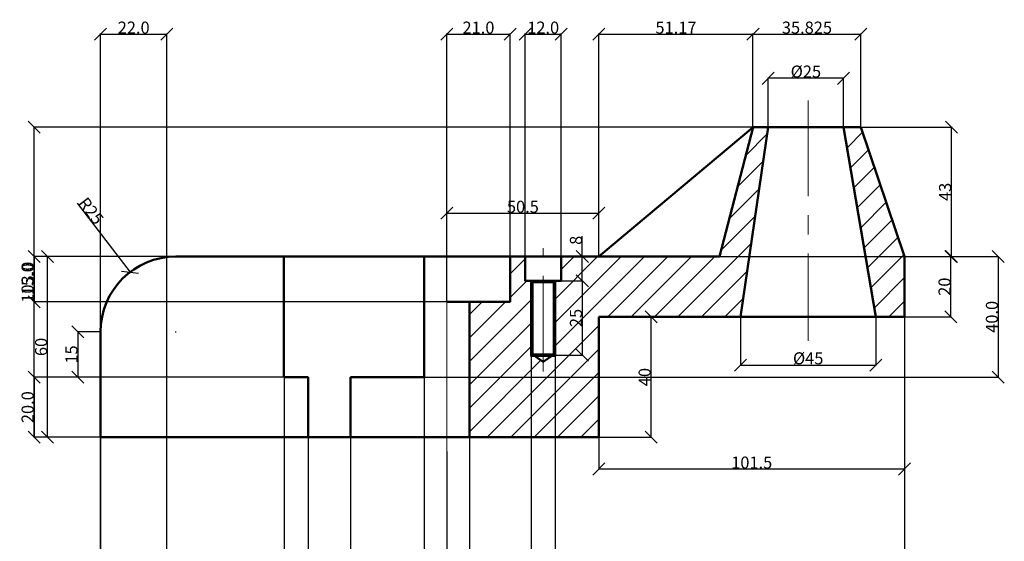
# Model space of a CAD drawing. Units: millimetres. Extents: x 263 to 611, y 50 to 522.
# Tile 5 of 5: x 284 to 611, y 349 to 522. Entities that reach past the tile are written whole.
import ezdxf

# ---------------------------------------------------------------- set-up
doc = ezdxf.new("R2010")
doc.units = ezdxf.units.MM
doc.header["$MEASUREMENT"] = 0
doc.linetypes.add('CENTER', pattern=[50.8, 31.75, -6.35, 6.35, -6.35])
for name, color, linetype, lineweight in [('M-CNTR', 1, 'CENTER', 18), ('M-DIMS', 2, 'Continuous', 25), ('M-HATC', 8, 'Continuous', 18), ('M-OUTL', 7, 'Continuous', 50)]:
    doc.layers.add(name, color=color, linetype=linetype, lineweight=lineweight)
doc.styles.get("Standard").update_dxf_attribs({"font": 'arial.ttf'})
doc.dimstyles.get("Standard").update_dxf_attribs({"dimtxt": 4, "dimasz": 4, "dimexe": 0.18, "dimexo": 0.0625, "dimgap": 0.09, "dimtad": 1, "dimdec": 0, "dimzin": 0, "dimdsep": 46, "dimtxsty": 'Standard', "dimblk": 'OBLIQUE', "dimcen": 0.09, "dimclre": 251, "dimadec": 0, "dimazin": 0, "dimtfac": 1, "dimtdec": 0, "dimtofl": 0, "dimtmove": 0, "dimatfit": 3, "dimfxl": 1, "dimtolj": 1, "dimtzin": 0, "dimarcsym": 0})

# ---------------------------------------------------------------- blocks, each defined once
blk = doc.blocks.new('_Oblique')
at = {"color": 0, "linetype": 'ByBlock', "lineweight": -2}
blk.add_line((-0.5, -0.5), (0.5, 0.5), dxfattribs=at)
blk = doc.blocks.new('*D37')
at = {"layer": 'Defpoints', "color": 0, "transparency": 16777216}
for p in [(476.6, 457.68), (426.1, 447.82), (476.6, 443.27)]:
    blk.add_point(p, dxfattribs=at)
at = {"layer": 'M-DIMS', "color": 0, "lineweight": -2, "transparency": 16777216}
for p, q in [((426.1, 447.88), (426.1, 457.86)), ((476.6, 443.34), (476.6, 457.86)), ((426.1, 457.68), (476.6, 457.68))]:
    blk.add_line(p, q, dxfattribs=at)
at = {"layer": 'M-DIMS', "color": 0, "lineweight": -2, "transparency": 16777216, "xscale": 4, "yscale": 4, "zscale": 4, "rotation": 180}
blk.add_blockref('_Oblique', (426.1, 457.68), dxfattribs=at)
at = {"layer": 'M-DIMS', "color": 0, "lineweight": -2, "transparency": 16777216, "xscale": 4, "yscale": 4, "zscale": 4}
blk.add_blockref('_Oblique', (476.6, 457.68), dxfattribs=at)
at = {"layer": 'M-DIMS', "color": 0, "transparency": 16777216, "insert": (451.35, 459.82), "char_height": 4, "attachment_point": 5}
blk.add_mtext('\\A1;50.5', dxfattribs=at)
blk = doc.blocks.new('*D38')
at = {"layer": 'Defpoints', "color": 0, "transparency": 16777216}
for p in [(464.1, 443.27), (471.09, 443.27), (464.1, 435.27)]:
    blk.add_point(p, dxfattribs=at)
at = {"layer": 'M-DIMS', "color": 0, "lineweight": -2, "transparency": 16777216}
for p, q in [((471.09, 443.27), (471.09, 450.09)), ((464.16, 443.27), (471.27, 443.27)), ((471.09, 435.27), (471.09, 443.27)), ((464.16, 435.27), (471.27, 435.27))]:
    blk.add_line(p, q, dxfattribs=at)
at = {"layer": 'M-DIMS', "color": 0, "lineweight": -2, "transparency": 16777216, "xscale": 4, "yscale": 4, "zscale": 4}
for p, rotation in [((471.09, 443.27), 90), ((471.09, 435.27), 270)]:
    blk.add_blockref('_Oblique', p, dxfattribs=dict(at, rotation=rotation))
at = {"layer": 'M-DIMS', "color": 0, "transparency": 16777216, "insert": (468.96, 448.68), "char_height": 4, "attachment_point": 5, "rotation": 90}
blk.add_mtext('\\A1;8', dxfattribs=at)
blk = doc.blocks.new('*D39')
at = {"layer": 'Defpoints', "color": 0, "transparency": 16777216}
for p in [(464.1, 435.27), (461.85, 410.52), (471.09, 410.52)]:
    blk.add_point(p, dxfattribs=at)
at = {"layer": 'M-DIMS', "color": 0, "lineweight": -2, "transparency": 16777216}
for p, q in [((464.16, 435.27), (471.27, 435.27)), ((471.09, 435.27), (471.09, 410.52)), ((461.91, 410.52), (471.27, 410.52))]:
    blk.add_line(p, q, dxfattribs=at)
at = {"layer": 'M-DIMS', "color": 0, "lineweight": -2, "transparency": 16777216, "xscale": 4, "yscale": 4, "zscale": 4}
for p, rotation in [((471.09, 435.27), 90), ((471.09, 410.52), 270)]:
    blk.add_blockref('_Oblique', p, dxfattribs=dict(at, rotation=rotation))
at = {"layer": 'M-DIMS', "color": 0, "transparency": 16777216, "insert": (468.96, 422.9), "char_height": 4, "attachment_point": 5, "rotation": 90}
blk.add_mtext('\\A1;25', dxfattribs=at)
blk = doc.blocks.new('*D40')
at = {"layer": 'Defpoints', "color": 0, "transparency": 16777216}
for p in [(487.01, 423.27), (493.93, 423.27), (476.6, 383.27)]:
    blk.add_point(p, dxfattribs=at)
at = {"layer": 'M-DIMS', "color": 0, "lineweight": -2, "transparency": 16777216}
for p, q in [((487.07, 423.27), (494.11, 423.27)), ((493.93, 383.27), (493.93, 423.27)), ((476.66, 383.27), (494.11, 383.27))]:
    blk.add_line(p, q, dxfattribs=at)
at = {"layer": 'M-DIMS', "color": 0, "lineweight": -2, "transparency": 16777216, "xscale": 4, "yscale": 4, "zscale": 4}
for p, rotation in [((493.93, 423.27), 90), ((493.93, 383.27), 270)]:
    blk.add_blockref('_Oblique', p, dxfattribs=dict(at, rotation=rotation))
at = {"layer": 'M-DIMS', "color": 0, "transparency": 16777216, "insert": (491.79, 403.27), "char_height": 4, "attachment_point": 5, "rotation": 90}
blk.add_mtext('\\A1;40', dxfattribs=at)
blk = doc.blocks.new('*D41')
at = {"layer": 'Defpoints', "color": 0, "transparency": 16777216}
for p in [(523.6, 423.27), (568.6, 423.27), (568.6, 407.25)]:
    blk.add_point(p, dxfattribs=at)
at = {"layer": 'M-DIMS', "color": 0, "lineweight": -2, "transparency": 16777216}
for p, q in [((523.6, 423.21), (523.6, 407.07)), ((568.6, 423.21), (568.6, 407.07)), ((523.6, 407.25), (568.6, 407.25))]:
    blk.add_line(p, q, dxfattribs=at)
at = {"layer": 'M-DIMS', "color": 0, "lineweight": -2, "transparency": 16777216, "xscale": 4, "yscale": 4, "zscale": 4, "rotation": 180}
blk.add_blockref('_Oblique', (523.6, 407.25), dxfattribs=at)
at = {"layer": 'M-DIMS', "color": 0, "lineweight": -2, "transparency": 16777216, "xscale": 4, "yscale": 4, "zscale": 4}
blk.add_blockref('_Oblique', (568.6, 407.25), dxfattribs=at)
at = {"layer": 'M-DIMS', "color": 0, "transparency": 16777216, "insert": (546.1, 409.5), "char_height": 4, "attachment_point": 5}
blk.add_mtext('\\A1;%%C45', dxfattribs=at)
blk = doc.blocks.new('*D42')
at = {"layer": 'Defpoints', "color": 0, "transparency": 16777216}
for p in [(578.1, 423.27), (476.6, 383.27), (578.1, 372.74)]:
    blk.add_point(p, dxfattribs=at)
at = {"layer": 'M-DIMS', "color": 0, "lineweight": -2, "transparency": 16777216}
for p, q in [((578.1, 423.21), (578.1, 372.56)), ((476.6, 383.21), (476.6, 372.56)), ((476.6, 372.74), (578.1, 372.74))]:
    blk.add_line(p, q, dxfattribs=at)
at = {"layer": 'M-DIMS', "color": 0, "lineweight": -2, "transparency": 16777216, "xscale": 4, "yscale": 4, "zscale": 4, "rotation": 180}
blk.add_blockref('_Oblique', (476.6, 372.74), dxfattribs=at)
at = {"layer": 'M-DIMS', "color": 0, "lineweight": -2, "transparency": 16777216, "xscale": 4, "yscale": 4, "zscale": 4}
blk.add_blockref('_Oblique', (578.1, 372.74), dxfattribs=at)
at = {"layer": 'M-DIMS', "color": 0, "transparency": 16777216, "insert": (527.35, 374.87), "char_height": 4, "attachment_point": 5}
blk.add_mtext('\\A1;101.5', dxfattribs=at)
blk = doc.blocks.new('*D43')
at = {"layer": 'Defpoints', "color": 0, "transparency": 16777216}
for p in [(578.1, 443.27), (593.52, 443.27), (578.1, 423.27)]:
    blk.add_point(p, dxfattribs=at)
at = {"layer": 'M-DIMS', "color": 0, "lineweight": -2, "transparency": 16777216}
for p, q in [((578.16, 443.27), (593.7, 443.27)), ((593.52, 423.27), (593.52, 443.27)), ((578.16, 423.27), (593.7, 423.27))]:
    blk.add_line(p, q, dxfattribs=at)
at = {"layer": 'M-DIMS', "color": 0, "lineweight": -2, "transparency": 16777216, "xscale": 4, "yscale": 4, "zscale": 4}
for p, rotation in [((593.52, 443.27), 90), ((593.52, 423.27), 270)]:
    blk.add_blockref('_Oblique', p, dxfattribs=dict(at, rotation=rotation))
at = {"layer": 'M-DIMS', "color": 0, "transparency": 16777216, "insert": (591.38, 433.27), "char_height": 4, "attachment_point": 5, "rotation": 90}
blk.add_mtext('\\A1;20', dxfattribs=at)
blk = doc.blocks.new('*D44')
at = {"layer": 'Defpoints', "color": 0, "transparency": 16777216}
for p in [(563.6, 486.27), (593.7, 486.27), (578.1, 443.27)]:
    blk.add_point(p, dxfattribs=at)
at = {"layer": 'M-DIMS', "color": 0, "lineweight": -2, "transparency": 16777216}
for p, q in [((563.66, 486.27), (593.88, 486.27)), ((593.7, 443.27), (593.7, 486.27)), ((578.16, 443.27), (593.88, 443.27))]:
    blk.add_line(p, q, dxfattribs=at)
at = {"layer": 'M-DIMS', "color": 0, "lineweight": -2, "transparency": 16777216, "xscale": 4, "yscale": 4, "zscale": 4}
for p, rotation in [((593.7, 486.27), 90), ((593.7, 443.27), 270)]:
    blk.add_blockref('_Oblique', p, dxfattribs=dict(at, rotation=rotation))
at = {"layer": 'M-DIMS', "color": 0, "transparency": 16777216, "insert": (591.56, 464.77), "char_height": 4, "attachment_point": 5, "rotation": 90}
blk.add_mtext('\\A1;43', dxfattribs=at)
blk = doc.blocks.new('*D45')
at = {"layer": 'Defpoints', "color": 0, "transparency": 16777216}
for p in [(532.83, 502.47), (532.83, 486.27), (557.83, 486.27)]:
    blk.add_point(p, dxfattribs=at)
at = {"layer": 'M-DIMS', "color": 0, "lineweight": -2, "transparency": 16777216}
for p, q in [((532.83, 486.34), (532.83, 502.65)), ((557.83, 502.47), (532.83, 502.47)), ((557.83, 486.34), (557.83, 502.65))]:
    blk.add_line(p, q, dxfattribs=at)
at = {"layer": 'M-DIMS', "color": 0, "lineweight": -2, "transparency": 16777216, "xscale": 4, "yscale": 4, "zscale": 4, "rotation": 180}
blk.add_blockref('_Oblique', (532.83, 502.47), dxfattribs=at)
at = {"layer": 'M-DIMS', "color": 0, "lineweight": -2, "transparency": 16777216, "xscale": 4, "yscale": 4, "zscale": 4}
blk.add_blockref('_Oblique', (557.83, 502.47), dxfattribs=at)
at = {"layer": 'M-DIMS', "color": 0, "transparency": 16777216, "insert": (545.33, 504.71), "char_height": 4, "attachment_point": 5}
blk.add_mtext('\\A1;%%C25', dxfattribs=at)
blk = doc.blocks.new('*D46')
at = {"layer": 'Defpoints', "color": 0, "transparency": 16777216}
for p in [(311.1, 418.27), (303.57, 403.27), (372.02, 403.27)]:
    blk.add_point(p, dxfattribs=at)
at = {"layer": 'M-DIMS', "color": 0, "lineweight": -2, "transparency": 16777216}
for p, q in [((311.04, 418.27), (303.39, 418.27)), ((303.57, 418.27), (303.57, 403.27)), ((371.95, 403.27), (303.39, 403.27))]:
    blk.add_line(p, q, dxfattribs=at)
at = {"layer": 'M-DIMS', "color": 0, "lineweight": -2, "transparency": 16777216, "xscale": 4, "yscale": 4, "zscale": 4}
for p, rotation in [((303.57, 418.27), 90), ((303.57, 403.27), 270)]:
    blk.add_blockref('_Oblique', p, dxfattribs=dict(at, rotation=rotation))
at = {"layer": 'M-DIMS', "color": 0, "transparency": 16777216, "insert": (301.44, 410.77), "char_height": 4, "attachment_point": 5, "rotation": 90}
blk.add_mtext('\\A1;15', dxfattribs=at)
blk = doc.blocks.new('*D47')
at = {"layer": 'Defpoints', "color": 0, "transparency": 16777216}
for p in [(293.47, 443.27), (336.1, 443.27), (311.1, 383.27)]:
    blk.add_point(p, dxfattribs=at)
at = {"layer": 'M-DIMS', "color": 0, "lineweight": -2, "transparency": 16777216}
for p, q in [((336.04, 443.27), (293.29, 443.27)), ((293.47, 383.27), (293.47, 443.27)), ((311.04, 383.27), (293.29, 383.27))]:
    blk.add_line(p, q, dxfattribs=at)
at = {"layer": 'M-DIMS', "color": 0, "lineweight": -2, "transparency": 16777216, "xscale": 4, "yscale": 4, "zscale": 4}
for p, rotation in [((293.47, 443.27), 90), ((293.47, 383.27), 270)]:
    blk.add_blockref('_Oblique', p, dxfattribs=dict(at, rotation=rotation))
at = {"layer": 'M-DIMS', "color": 0, "transparency": 16777216, "insert": (291.34, 413.27), "char_height": 4, "attachment_point": 5, "rotation": 90}
blk.add_mtext('\\A1;60', dxfattribs=at)
blk = doc.blocks.new('*D48')
at = {"layer": 'Defpoints', "color": 0, "transparency": 16777216}
for p in [(320.88, 438.1), (336.1, 418.27)]:
    blk.add_point(p, dxfattribs=at)
at = {"layer": 'M-DIMS', "color": 0, "lineweight": -2, "transparency": 16777216}
for p, q in [((303.29, 461.02), (320.88, 438.1)), ((336.01, 418.27), (336.19, 418.27)), ((336.1, 418.18), (336.1, 418.36))]:
    blk.add_line(p, q, dxfattribs=at)
at = {"layer": 'M-DIMS', "color": 0, "lineweight": -2, "transparency": 16777216, "xscale": 4, "yscale": 4, "zscale": 4, "rotation": 307.5089199035373}
blk.add_blockref('_Oblique', (320.88, 438.1), dxfattribs=at)
at = {"layer": 'M-DIMS', "color": 0, "transparency": 16777216, "insert": (307.95, 458.44), "char_height": 4, "attachment_point": 5, "rotation": 307.5089}
blk.add_mtext('\\A1;R25', dxfattribs=at)
blk = doc.blocks.new('*D52')
at = {"layer": 'Defpoints', "color": 0, "transparency": 16777216}
for p in [(333.1, 517.18), (333.1, 226.08), (311.1, 223.08)]:
    blk.add_point(p, dxfattribs=at)
at = {"layer": 'M-DIMS', "color": 251, "lineweight": -2, "transparency": 16777216}
for p, q in [((311.1, 223.14), (311.1, 517.36)), ((333.1, 226.14), (333.1, 517.36))]:
    blk.add_line(p, q, dxfattribs=at)
at = {"layer": 'M-DIMS', "color": 0, "lineweight": -2, "transparency": 16777216}
blk.add_line((311.1, 517.18), (333.1, 517.18), dxfattribs=at)
at = {"layer": 'M-DIMS', "color": 0, "lineweight": -2, "transparency": 16777216, "xscale": 4, "yscale": 4, "zscale": 4, "rotation": 180}
blk.add_blockref('_Oblique', (311.1, 517.18), dxfattribs=at)
at = {"layer": 'M-DIMS', "color": 0, "lineweight": -2, "transparency": 16777216, "xscale": 4, "yscale": 4, "zscale": 4}
blk.add_blockref('_Oblique', (333.1, 517.18), dxfattribs=at)
at = {"layer": 'M-DIMS', "color": 0, "transparency": 16777216, "insert": (322.1, 519.31), "char_height": 4, "attachment_point": 5}
blk.add_mtext('\\A1;22.0', dxfattribs=at)
blk = doc.blocks.new('*D53')
at = {"layer": 'Defpoints', "color": 0, "transparency": 16777216}
for p in [(578.1, 423.27), (311.1, 383.27), (578.1, 52.26)]:
    blk.add_point(p, dxfattribs=at)
at = {"layer": 'M-DIMS', "color": 251, "lineweight": -2, "transparency": 16777216}
for p, q in [((578.1, 423.21), (578.1, 52.08)), ((311.1, 383.21), (311.1, 52.08))]:
    blk.add_line(p, q, dxfattribs=at)
at = {"layer": 'M-DIMS', "color": 0, "lineweight": -2, "transparency": 16777216}
blk.add_line((311.1, 52.26), (578.1, 52.26), dxfattribs=at)
at = {"layer": 'M-DIMS', "color": 0, "lineweight": -2, "transparency": 16777216, "xscale": 4, "yscale": 4, "zscale": 4, "rotation": 180}
blk.add_blockref('_Oblique', (311.1, 52.26), dxfattribs=at)
at = {"layer": 'M-DIMS', "color": 0, "lineweight": -2, "transparency": 16777216, "xscale": 4, "yscale": 4, "zscale": 4}
blk.add_blockref('_Oblique', (578.1, 52.26), dxfattribs=at)
at = {"layer": 'M-DIMS', "color": 0, "transparency": 16777216, "insert": (444.6, 54.39), "char_height": 4, "attachment_point": 5}
blk.add_mtext('\\A1;267.0', dxfattribs=at)
blk = doc.blocks.new('*D54')
at = {"layer": 'Defpoints', "color": 0, "transparency": 16777216}
for p in [(289, 486.27), (527.77, 486.27), (311.1, 383.27)]:
    blk.add_point(p, dxfattribs=at)
at = {"layer": 'M-DIMS', "color": 251, "lineweight": -2, "transparency": 16777216}
for p, q in [((527.71, 486.27), (288.82, 486.27)), ((311.04, 383.27), (288.82, 383.27))]:
    blk.add_line(p, q, dxfattribs=at)
at = {"layer": 'M-DIMS', "color": 0, "lineweight": -2, "transparency": 16777216}
blk.add_line((289, 383.27), (289, 486.27), dxfattribs=at)
at = {"layer": 'M-DIMS', "color": 0, "lineweight": -2, "transparency": 16777216, "xscale": 4, "yscale": 4, "zscale": 4}
for p, rotation in [((289, 486.27), 90), ((289, 383.27), 270)]:
    blk.add_blockref('_Oblique', p, dxfattribs=dict(at, rotation=rotation))
at = {"layer": 'M-DIMS', "color": 0, "transparency": 16777216, "insert": (286.87, 434.77), "char_height": 4, "attachment_point": 5, "rotation": 90}
blk.add_mtext('\\A1;103.0', dxfattribs=at)
blk = doc.blocks.new('*D55')
at = {"layer": 'Defpoints', "color": 0, "transparency": 16777216}
for p in [(464.1, 517.18), (452.1, 443.27), (464.1, 443.27)]:
    blk.add_point(p, dxfattribs=at)
at = {"layer": 'M-DIMS', "color": 251, "lineweight": -2, "transparency": 16777216}
for p, q in [((452.1, 443.34), (452.1, 517.36)), ((464.1, 443.34), (464.1, 517.36))]:
    blk.add_line(p, q, dxfattribs=at)
at = {"layer": 'M-DIMS', "color": 0, "lineweight": -2, "transparency": 16777216}
blk.add_line((452.1, 517.18), (464.1, 517.18), dxfattribs=at)
at = {"layer": 'M-DIMS', "color": 0, "lineweight": -2, "transparency": 16777216, "xscale": 4, "yscale": 4, "zscale": 4, "rotation": 180}
blk.add_blockref('_Oblique', (452.1, 517.18), dxfattribs=at)
at = {"layer": 'M-DIMS', "color": 0, "lineweight": -2, "transparency": 16777216, "xscale": 4, "yscale": 4, "zscale": 4}
blk.add_blockref('_Oblique', (464.1, 517.18), dxfattribs=at)
at = {"layer": 'M-DIMS', "color": 0, "transparency": 16777216, "insert": (458.1, 519.31), "char_height": 4, "attachment_point": 5}
blk.add_mtext('\\A1;12.0', dxfattribs=at)
blk = doc.blocks.new('*D56')
at = {"layer": 'Defpoints', "color": 0, "transparency": 16777216}
for p in [(454.1, 410.27), (462.1, 410.27), (462.1, 52.26)]:
    blk.add_point(p, dxfattribs=at)
at = {"layer": 'M-DIMS', "color": 251, "lineweight": -2, "transparency": 16777216}
for p, q in [((454.1, 410.21), (454.1, 52.08)), ((462.1, 410.21), (462.1, 52.08))]:
    blk.add_line(p, q, dxfattribs=at)
at = {"layer": 'M-DIMS', "color": 0, "lineweight": -2, "transparency": 16777216}
blk.add_line((454.1, 52.26), (462.1, 52.26), dxfattribs=at)
at = {"layer": 'M-DIMS', "color": 0, "lineweight": -2, "transparency": 16777216, "xscale": 4, "yscale": 4, "zscale": 4, "rotation": 180}
blk.add_blockref('_Oblique', (454.1, 52.26), dxfattribs=at)
at = {"layer": 'M-DIMS', "color": 0, "lineweight": -2, "transparency": 16777216, "xscale": 4, "yscale": 4, "zscale": 4}
blk.add_blockref('_Oblique', (462.1, 52.26), dxfattribs=at)
at = {"layer": 'M-DIMS', "color": 0, "transparency": 16777216, "insert": (458.1, 54.39), "char_height": 4, "attachment_point": 5}
blk.add_mtext('\\A1;8.0', dxfattribs=at)
blk = doc.blocks.new('*D57')
at = {"layer": 'Defpoints', "color": 0, "transparency": 16777216}
for p in [(372.02, 403.27), (311.1, 383.27), (372.02, 52.26)]:
    blk.add_point(p, dxfattribs=at)
at = {"layer": 'M-DIMS', "color": 251, "lineweight": -2, "transparency": 16777216}
for p, q in [((372.02, 403.21), (372.02, 52.08)), ((311.1, 383.21), (311.1, 52.08))]:
    blk.add_line(p, q, dxfattribs=at)
at = {"layer": 'M-DIMS', "color": 0, "lineweight": -2, "transparency": 16777216}
blk.add_line((311.1, 52.26), (372.02, 52.26), dxfattribs=at)
at = {"layer": 'M-DIMS', "color": 0, "lineweight": -2, "transparency": 16777216, "xscale": 4, "yscale": 4, "zscale": 4, "rotation": 180}
blk.add_blockref('_Oblique', (311.1, 52.26), dxfattribs=at)
at = {"layer": 'M-DIMS', "color": 0, "lineweight": -2, "transparency": 16777216, "xscale": 4, "yscale": 4, "zscale": 4}
blk.add_blockref('_Oblique', (372.02, 52.26), dxfattribs=at)
at = {"layer": 'M-DIMS', "color": 0, "transparency": 16777216, "insert": (341.56, 54.39), "char_height": 4, "attachment_point": 5}
blk.add_mtext('\\A1;60.92', dxfattribs=at)
blk = doc.blocks.new('*D58')
at = {"layer": 'Defpoints', "color": 0, "transparency": 16777216}
for p in [(372.02, 403.27), (380, 383.27), (380, 52.26)]:
    blk.add_point(p, dxfattribs=at)
at = {"layer": 'M-DIMS', "color": 251, "lineweight": -2, "transparency": 16777216}
for p, q in [((372.02, 403.21), (372.02, 52.08)), ((380, 383.21), (380, 52.08))]:
    blk.add_line(p, q, dxfattribs=at)
at = {"layer": 'M-DIMS', "color": 0, "lineweight": -2, "transparency": 16777216}
for p, q in [((372.02, 52.26), (380, 52.26)), ((380, 52.26), (397.64, 52.26))]:
    blk.add_line(p, q, dxfattribs=at)
at = {"layer": 'M-DIMS', "color": 0, "lineweight": -2, "transparency": 16777216, "xscale": 4, "yscale": 4, "zscale": 4, "rotation": 180}
blk.add_blockref('_Oblique', (372.02, 52.26), dxfattribs=at)
at = {"layer": 'M-DIMS', "color": 0, "lineweight": -2, "transparency": 16777216, "xscale": 4, "yscale": 4, "zscale": 4}
blk.add_blockref('_Oblique', (380, 52.26), dxfattribs=at)
at = {"layer": 'M-DIMS', "color": 0, "transparency": 16777216, "insert": (390.82, 54.39), "char_height": 4, "attachment_point": 5}
blk.add_mtext('\\A1;7.986', dxfattribs=at)
blk = doc.blocks.new('*D59')
at = {"layer": 'Defpoints', "color": 0, "transparency": 16777216}
for p in [(380, 383.27), (394.1, 383.27), (394.1, 52.26)]:
    blk.add_point(p, dxfattribs=at)
at = {"layer": 'M-DIMS', "color": 251, "lineweight": -2, "transparency": 16777216}
for p, q in [((380, 383.21), (380, 52.08)), ((394.1, 383.21), (394.1, 52.08))]:
    blk.add_line(p, q, dxfattribs=at)
at = {"layer": 'M-DIMS', "color": 0, "lineweight": -2, "transparency": 16777216}
for p, q in [((380, 52.26), (394.1, 52.26)), ((394.1, 52.26), (414.52, 52.26))]:
    blk.add_line(p, q, dxfattribs=at)
at = {"layer": 'M-DIMS', "color": 0, "lineweight": -2, "transparency": 16777216, "xscale": 4, "yscale": 4, "zscale": 4, "rotation": 180}
blk.add_blockref('_Oblique', (380, 52.26), dxfattribs=at)
at = {"layer": 'M-DIMS', "color": 0, "lineweight": -2, "transparency": 16777216, "xscale": 4, "yscale": 4, "zscale": 4}
blk.add_blockref('_Oblique', (394.1, 52.26), dxfattribs=at)
at = {"layer": 'M-DIMS', "color": 0, "transparency": 16777216, "insert": (406.31, 54.39), "char_height": 4, "attachment_point": 5}
blk.add_mtext('\\A1;14.098', dxfattribs=at)
blk = doc.blocks.new('*D60')
at = {"layer": 'Defpoints', "color": 0, "transparency": 16777216}
for p in [(418.6, 403.27), (394.1, 383.27), (418.6, 52.26)]:
    blk.add_point(p, dxfattribs=at)
at = {"layer": 'M-DIMS', "color": 251, "lineweight": -2, "transparency": 16777216}
for p, q in [((418.6, 403.21), (418.6, 52.08)), ((394.1, 383.21), (394.1, 52.08))]:
    blk.add_line(p, q, dxfattribs=at)
at = {"layer": 'M-DIMS', "color": 0, "lineweight": -2, "transparency": 16777216}
blk.add_line((394.1, 52.26), (418.6, 52.26), dxfattribs=at)
at = {"layer": 'M-DIMS', "color": 0, "lineweight": -2, "transparency": 16777216, "xscale": 4, "yscale": 4, "zscale": 4, "rotation": 180}
blk.add_blockref('_Oblique', (394.1, 52.26), dxfattribs=at)
at = {"layer": 'M-DIMS', "color": 0, "lineweight": -2, "transparency": 16777216, "xscale": 4, "yscale": 4, "zscale": 4}
blk.add_blockref('_Oblique', (418.6, 52.26), dxfattribs=at)
at = {"layer": 'M-DIMS', "color": 0, "transparency": 16777216, "insert": (406.35, 54.39), "char_height": 4, "attachment_point": 5}
blk.add_mtext('\\A1;24.5', dxfattribs=at)
blk = doc.blocks.new('*D61')
at = {"layer": 'Defpoints', "color": 0, "transparency": 16777216}
for p in [(418.6, 403.27), (426.1, 378.63), (426.1, 52.26)]:
    blk.add_point(p, dxfattribs=at)
at = {"layer": 'M-DIMS', "color": 251, "lineweight": -2, "transparency": 16777216}
for p, q in [((418.6, 403.21), (418.6, 52.08)), ((426.1, 378.57), (426.1, 52.08))]:
    blk.add_line(p, q, dxfattribs=at)
at = {"layer": 'M-DIMS', "color": 0, "lineweight": -2, "transparency": 16777216}
blk.add_line((418.6, 52.26), (426.1, 52.26), dxfattribs=at)
at = {"layer": 'M-DIMS', "color": 0, "lineweight": -2, "transparency": 16777216, "xscale": 4, "yscale": 4, "zscale": 4, "rotation": 180}
blk.add_blockref('_Oblique', (418.6, 52.26), dxfattribs=at)
at = {"layer": 'M-DIMS', "color": 0, "lineweight": -2, "transparency": 16777216, "xscale": 4, "yscale": 4, "zscale": 4}
blk.add_blockref('_Oblique', (426.1, 52.26), dxfattribs=at)
at = {"layer": 'M-DIMS', "color": 0, "transparency": 16777216, "insert": (422.35, 54.38), "char_height": 4, "attachment_point": 5}
blk.add_mtext('\\A1;7.5', dxfattribs=at)
blk = doc.blocks.new('*D62')
at = {"layer": 'Defpoints', "color": 0, "transparency": 16777216}
for p in [(433.6, 383.27), (426.1, 378.63), (433.6, 52.26)]:
    blk.add_point(p, dxfattribs=at)
at = {"layer": 'M-DIMS', "color": 251, "lineweight": -2, "transparency": 16777216}
for p, q in [((433.6, 383.21), (433.6, 52.08)), ((426.1, 378.57), (426.1, 52.08))]:
    blk.add_line(p, q, dxfattribs=at)
at = {"layer": 'M-DIMS', "color": 0, "lineweight": -2, "transparency": 16777216}
blk.add_line((426.1, 52.26), (433.6, 52.26), dxfattribs=at)
at = {"layer": 'M-DIMS', "color": 0, "lineweight": -2, "transparency": 16777216, "xscale": 4, "yscale": 4, "zscale": 4, "rotation": 180}
blk.add_blockref('_Oblique', (426.1, 52.26), dxfattribs=at)
at = {"layer": 'M-DIMS', "color": 0, "lineweight": -2, "transparency": 16777216, "xscale": 4, "yscale": 4, "zscale": 4}
blk.add_blockref('_Oblique', (433.6, 52.26), dxfattribs=at)
at = {"layer": 'M-DIMS', "color": 0, "transparency": 16777216, "insert": (429.85, 54.38), "char_height": 4, "attachment_point": 5}
blk.add_mtext('\\A1;7.5', dxfattribs=at)
blk = doc.blocks.new('*D63')
at = {"layer": 'Defpoints', "color": 0, "transparency": 16777216}
for p in [(418.6, 443.27), (418.6, 403.27), (609.23, 403.27)]:
    blk.add_point(p, dxfattribs=at)
at = {"layer": 'M-DIMS', "color": 251, "lineweight": -2, "transparency": 16777216}
for p, q in [((418.66, 443.27), (609.41, 443.27)), ((418.66, 403.27), (609.41, 403.27))]:
    blk.add_line(p, q, dxfattribs=at)
at = {"layer": 'M-DIMS', "color": 0, "lineweight": -2, "transparency": 16777216}
blk.add_line((609.23, 443.27), (609.23, 403.27), dxfattribs=at)
at = {"layer": 'M-DIMS', "color": 0, "lineweight": -2, "transparency": 16777216, "xscale": 4, "yscale": 4, "zscale": 4}
for p, rotation in [((609.23, 443.27), 90), ((609.23, 403.27), 270)]:
    blk.add_blockref('_Oblique', p, dxfattribs=dict(at, rotation=rotation))
at = {"layer": 'M-DIMS', "color": 0, "transparency": 16777216, "insert": (607.1, 423.27), "char_height": 4, "attachment_point": 5, "rotation": 90}
blk.add_mtext('\\A1;40.0', dxfattribs=at)
blk = doc.blocks.new('*D64')
at = {"layer": 'Defpoints', "color": 0, "transparency": 16777216}
for p in [(380, 403.27), (289, 383.27), (380, 383.27)]:
    blk.add_point(p, dxfattribs=at)
at = {"layer": 'M-DIMS', "color": 251, "lineweight": -2, "transparency": 16777216}
for p, q in [((379.94, 403.27), (288.82, 403.27)), ((379.94, 383.27), (288.82, 383.27))]:
    blk.add_line(p, q, dxfattribs=at)
at = {"layer": 'M-DIMS', "color": 0, "lineweight": -2, "transparency": 16777216}
blk.add_line((289, 403.27), (289, 383.27), dxfattribs=at)
at = {"layer": 'M-DIMS', "color": 0, "lineweight": -2, "transparency": 16777216, "xscale": 4, "yscale": 4, "zscale": 4}
for p, rotation in [((289, 403.27), 90), ((289, 383.27), 270)]:
    blk.add_blockref('_Oblique', p, dxfattribs=dict(at, rotation=rotation))
at = {"layer": 'M-DIMS', "color": 0, "transparency": 16777216, "insert": (286.87, 393.27), "char_height": 4, "attachment_point": 5, "rotation": 90}
blk.add_mtext('\\A1;20.0', dxfattribs=at)
blk = doc.blocks.new('*D65')
at = {"layer": 'Defpoints', "color": 0, "transparency": 16777216}
for p in [(447.1, 517.18), (426.1, 428.27), (447.1, 428.27)]:
    blk.add_point(p, dxfattribs=at)
at = {"layer": 'M-DIMS', "color": 251, "lineweight": -2, "transparency": 16777216}
for p, q in [((426.1, 428.34), (426.1, 517.36)), ((447.1, 428.34), (447.1, 517.36))]:
    blk.add_line(p, q, dxfattribs=at)
at = {"layer": 'M-DIMS', "color": 0, "lineweight": -2, "transparency": 16777216}
blk.add_line((426.1, 517.18), (447.1, 517.18), dxfattribs=at)
at = {"layer": 'M-DIMS', "color": 0, "lineweight": -2, "transparency": 16777216, "xscale": 4, "yscale": 4, "zscale": 4, "rotation": 180}
blk.add_blockref('_Oblique', (426.1, 517.18), dxfattribs=at)
at = {"layer": 'M-DIMS', "color": 0, "lineweight": -2, "transparency": 16777216, "xscale": 4, "yscale": 4, "zscale": 4}
blk.add_blockref('_Oblique', (447.1, 517.18), dxfattribs=at)
at = {"layer": 'M-DIMS', "color": 0, "transparency": 16777216, "insert": (436.6, 519.31), "char_height": 4, "attachment_point": 5}
blk.add_mtext('\\A1;21.0', dxfattribs=at)
blk = doc.blocks.new('*D66')
at = {"layer": 'Defpoints', "color": 0, "transparency": 16777216}
for p in [(447.1, 443.27), (289, 428.27), (447.1, 428.27)]:
    blk.add_point(p, dxfattribs=at)
at = {"layer": 'M-DIMS', "color": 251, "lineweight": -2, "transparency": 16777216}
for p, q in [((447.03, 443.27), (288.82, 443.27)), ((447.03, 428.27), (288.82, 428.27))]:
    blk.add_line(p, q, dxfattribs=at)
at = {"layer": 'M-DIMS', "color": 0, "lineweight": -2, "transparency": 16777216}
blk.add_line((289, 443.27), (289, 428.27), dxfattribs=at)
at = {"layer": 'M-DIMS', "color": 0, "lineweight": -2, "transparency": 16777216, "xscale": 4, "yscale": 4, "zscale": 4}
for p, rotation in [((289, 443.27), 90), ((289, 428.27), 270)]:
    blk.add_blockref('_Oblique', p, dxfattribs=dict(at, rotation=rotation))
at = {"layer": 'M-DIMS', "color": 0, "transparency": 16777216, "insert": (286.87, 435.77), "char_height": 4, "attachment_point": 5, "rotation": 90}
blk.add_mtext('\\A1;15.0', dxfattribs=at)
blk = doc.blocks.new('*D67')
at = {"layer": 'Defpoints', "color": 0, "transparency": 16777216}
for p in [(527.77, 517.18), (527.77, 486.27), (476.6, 443.27)]:
    blk.add_point(p, dxfattribs=at)
at = {"layer": 'M-DIMS', "color": 251, "lineweight": -2, "transparency": 16777216}
for p, q in [((476.6, 443.34), (476.6, 517.36)), ((527.77, 486.34), (527.77, 517.36))]:
    blk.add_line(p, q, dxfattribs=at)
at = {"layer": 'M-DIMS', "color": 0, "lineweight": -2, "transparency": 16777216}
blk.add_line((476.6, 517.18), (527.77, 517.18), dxfattribs=at)
at = {"layer": 'M-DIMS', "color": 0, "lineweight": -2, "transparency": 16777216, "xscale": 4, "yscale": 4, "zscale": 4, "rotation": 180}
blk.add_blockref('_Oblique', (476.6, 517.18), dxfattribs=at)
at = {"layer": 'M-DIMS', "color": 0, "lineweight": -2, "transparency": 16777216, "xscale": 4, "yscale": 4, "zscale": 4}
blk.add_blockref('_Oblique', (527.77, 517.18), dxfattribs=at)
at = {"layer": 'M-DIMS', "color": 0, "transparency": 16777216, "insert": (502.19, 519.31), "char_height": 4, "attachment_point": 5}
blk.add_mtext('\\A1;51.17', dxfattribs=at)
blk = doc.blocks.new('*D68')
at = {"layer": 'Defpoints', "color": 0, "transparency": 16777216}
for p in [(563.6, 517.18), (527.77, 486.27), (563.6, 486.27)]:
    blk.add_point(p, dxfattribs=at)
at = {"layer": 'M-DIMS', "color": 251, "lineweight": -2, "transparency": 16777216}
for p, q in [((527.77, 486.34), (527.77, 517.36)), ((563.6, 486.34), (563.6, 517.36))]:
    blk.add_line(p, q, dxfattribs=at)
at = {"layer": 'M-DIMS', "color": 0, "lineweight": -2, "transparency": 16777216}
blk.add_line((527.77, 517.18), (563.6, 517.18), dxfattribs=at)
at = {"layer": 'M-DIMS', "color": 0, "lineweight": -2, "transparency": 16777216, "xscale": 4, "yscale": 4, "zscale": 4, "rotation": 180}
blk.add_blockref('_Oblique', (527.77, 517.18), dxfattribs=at)
at = {"layer": 'M-DIMS', "color": 0, "lineweight": -2, "transparency": 16777216, "xscale": 4, "yscale": 4, "zscale": 4}
blk.add_blockref('_Oblique', (563.6, 517.18), dxfattribs=at)
at = {"layer": 'M-DIMS', "color": 0, "transparency": 16777216, "insert": (545.69, 519.31), "char_height": 4, "attachment_point": 5}
blk.add_mtext('\\A1;35.825', dxfattribs=at)

msp = doc.modelspace()

# ---------------------------------------------------------------- hatches: boundary and pattern name
at = {"layer": 'M-HATC'}
h = msp.add_hatch(dxfattribs=at)
h.set_pattern_fill('ANSI31', color=256, scale=44)
h.set_pattern_definition([(45, (0, 91.5403), (-3.889087, 3.889087), [])])
h.paths.add_polyline_path([(476.5988, 383.2727), (476.5988, 423.2727), (523.5988, 423.2727), (532.8271, 486.2727), (527.7737, 486.2727), (516.6719, 443.2727), (464.0988, 443.2727), (464.0988, 435.2727), (462.0988, 435.2727), (462.0988, 410.2727), (460.8811, 410.2727), (458.0988, 408.3344), (455.3165, 410.2727), (454.0988, 410.2727), (454.0988, 435.2727), (452.0988, 435.2727), (452.0988, 443.2727), (447.0973, 443.2727), (447.0973, 428.2727), (433.5988, 428.2727), (433.5988, 383.2727)])
h.paths.add_polyline_path([(568.5988, 423.2727), (578.0988, 423.2727), (578.0988, 443.2727), (563.5988, 486.2727), (557.8271, 486.2727)])

# ---------------------------------------------------------------- linework, layer by layer
at = {"layer": 'M-CNTR'}
for p, q in [((546.0988, 495.0806), (546.0988, 415.3229)), ((426.0988, 378.6323), (426.0988, 447.8203)), ((458.0988, 405.1608), (458.0988, 446.1103)), ((426.0988, 403.2727), (426.0988, 443.2727)), ((426.0988, 403.2727), (426.0988, 443.2727))]:
    msp.add_line(p, q, dxfattribs=at)
at = {"layer": 'M-OUTL'}
for p, q in [((476.5988, 443.2727), (527.7737, 486.2727)), ((527.7737, 486.2727), (516.6719, 443.2727)), ((532.8271, 486.2727), (523.5988, 423.2727)), ((527.7737, 486.2727), (563.5988, 486.2727)), ((532.8271, 486.2727), (557.8271, 486.2727)), ((557.8271, 486.2727), (568.5988, 423.2727)), ((563.5988, 486.2727), (578.0988, 443.2727)), ((336.0988, 443.2727), (516.6719, 443.2727)), ((372.0156, 403.2727), (372.0156, 443.2727)), ((418.5988, 443.2727), (418.5988, 403.2727)), ((447.0973, 443.2727), (447.0973, 428.2727)), ((578.0988, 423.2727), (578.0988, 443.2727)), ((426.0988, 428.2727), (447.0973, 428.2727)), ((433.5988, 428.2727), (433.5988, 383.2727)), ((476.5988, 423.2727), (578.0988, 423.2727)), ((476.5988, 423.2727), (476.5988, 383.2727)), ((311.0988, 383.2727), (311.0988, 418.2727)), ((454.0988, 410.2727), (454.5988, 410.7727)), ((454.5988, 410.7727), (458.0988, 408.3344)), ((458.0988, 408.3344), (461.5988, 410.7727)), ((461.5988, 410.7727), (462.0988, 410.2727)), ((372.0156, 403.2727), (380.0011, 403.2727)), ((380.0011, 403.2727), (380.0011, 383.2727)), ((394.0988, 403.2727), (394.0988, 383.2727)), ((394.0988, 403.2727), (418.5988, 403.2727)), ((311.0988, 383.2727), (476.5988, 383.2727))]:
    msp.add_line(p, q, dxfattribs=at)
for points in [[(452.0988, 443.2727), (464.0988, 443.2727), (464.0988, 435.2727), (452.0988, 435.2727)], [(454.0988, 435.2727), (462.0988, 435.2727), (462.0988, 410.2727), (454.0988, 410.2727)], [(454.5988, 434.7727), (461.5988, 434.7727), (461.5988, 410.7727), (454.5988, 410.7727)]]:
    msp.add_lwpolyline(points, close=True, dxfattribs=at)
msp.add_arc((336.0988, 418.2727), 25, 90, 180, dxfattribs=at)

# ---------------------------------------------------------------- dimensions: what is measured, and where the dimension line sits
at = {"layer": 'M-DIMS'}
for base, p1, p2, override, picture, middle in [((333.0988, 517.1806), (311.0988, 223.0815), (333.0988, 226.0815), {"dimdec": 1, "dimlfac": 1, "dimrnd": 0, "dimzin": 0, "dimdsep": 46, "dimlunit": 2}, '*D52', (322.0988, 519.3128)), ((447.0973, 517.1806), (426.0988, 428.2727), (447.0973, 428.2727), {"dimdec": 1, "dimlfac": 1, "dimrnd": 0, "dimzin": 0, "dimdsep": 46, "dimlunit": 2}, '*D65', (436.5981, 519.3128)), ((464.0988, 517.1806), (452.0988, 443.2727), (464.0988, 443.2727), {"dimdec": 1, "dimlfac": 1, "dimrnd": 0, "dimzin": 0, "dimdsep": 46, "dimlunit": 2}, '*D55', (458.0988, 519.3128)), ((527.7737, 517.1806), (476.5988, 443.2727), (527.7737, 486.2727), {"dimdec": 2, "dimlfac": 1, "dimrnd": 0, "dimzin": 0, "dimdsep": 46, "dimlunit": 2}, '*D67', (502.1863, 519.3128)), ((563.5988, 517.1806), (527.7737, 486.2727), (563.5988, 486.2727), {"dimdec": 3, "dimlfac": 1, "dimrnd": 0, "dimzin": 0, "dimdsep": 46, "dimlunit": 2}, '*D68', (545.6863, 519.3142)), ((476.5988, 457.6837), (426.0988, 447.8203), (476.5988, 443.2727), {"dimdec": 1, "dimclrd": 0, "dimclre": 0, "dimclrt": 0}, '*D37', (451.3488, 459.816)), ((578.0988, 52.2557), (311.0988, 383.2727), (578.0988, 423.2727), {"dimdec": 1, "dimlfac": 1, "dimrnd": 0, "dimzin": 0, "dimdsep": 46, "dimlunit": 2}, '*D53', (444.5988, 54.388)), ((578.0988, 372.741), (476.5988, 383.2727), (578.0988, 423.2727), {"dimdec": 1, "dimclrd": 0, "dimclre": 0, "dimclrt": 0}, '*D42', (527.3488, 374.8733)), ((462.0988, 52.2557), (454.0988, 410.2727), (462.0988, 410.2727), {"dimdec": 1, "dimlfac": 1, "dimrnd": 0, "dimzin": 0, "dimdsep": 46, "dimlunit": 2}, '*D56', (458.0988, 54.388)), ((372.0156, 52.2557), (311.0988, 383.2727), (372.0156, 403.2727), {"dimdec": 2, "dimlfac": 1, "dimrnd": 0, "dimzin": 0, "dimdsep": 46, "dimlunit": 2}, '*D57', (341.5572, 54.388)), ((380.00111, 52.25572), (372.01556, 403.2727), (380.00111, 383.2727), {"dimdec": 3, "dimlfac": 1, "dimrnd": 0, "dimzin": 0, "dimdsep": 46, "dimlunit": 2}, '*D58', (390.82235, 54.38801)), ((418.5988, 52.2557), (394.0988, 383.2727), (418.5988, 403.2727), {"dimdec": 1, "dimlfac": 1, "dimrnd": 0, "dimzin": 0, "dimdsep": 46, "dimlunit": 2}, '*D60', (406.3488, 54.388)), ((426.0988, 52.2557), (418.5988, 403.2727), (426.0988, 378.6323), {"dimdec": 1, "dimlfac": 1, "dimrnd": 0, "dimzin": 0, "dimdsep": 46, "dimlunit": 2}, '*D61', (422.3488, 54.3798)), ((394.0988, 52.2557), (380.0011, 383.2727), (394.0988, 383.2727), {"dimdec": 3, "dimlfac": 1, "dimrnd": 0, "dimzin": 0, "dimdsep": 46, "dimlunit": 2}, '*D59', (406.3075, 54.388)), ((433.5988, 52.2557), (426.0988, 378.6323), (433.5988, 383.2727), {"dimdec": 1, "dimlfac": 1, "dimrnd": 0, "dimzin": 0, "dimdsep": 46, "dimlunit": 2}, '*D62', (429.8488, 54.3798))]:
    dim = msp.add_linear_dim(base=base, p1=p1, p2=p2, dimstyle='Standard', override=override, dxfattribs=at)
    dim.commit()
    dim.dimension.update_dxf_attribs({"geometry": picture, "text_midpoint": middle})
for base, p1, p2, picture, middle in [((532.8271, 502.4685), (557.8271, 486.2727), (532.8271, 486.2727), '*D45', (545.3271, 504.7126)), ((568.5988, 407.2536), (523.5988, 423.2727), (568.5988, 423.2727), '*D41', (546.0988, 409.4978))]:
    dim = msp.add_linear_dim(base=base, p1=p1, p2=p2, text='%%C<>', dimstyle='Standard', override={"dimclrd": 0, "dimclre": 0, "dimclrt": 0}, dxfattribs=at)
    dim.commit()
    dim.dimension.update_dxf_attribs({"geometry": picture, "text_midpoint": middle})
for base, p1, p2, override, picture, middle in [((288.9988, 486.2727), (311.0988, 383.2727), (527.7737, 486.2727), {"dimdec": 1, "dimlfac": 1, "dimrnd": 0, "dimzin": 0, "dimdsep": 46, "dimlunit": 2}, '*D54', (286.8652, 434.7727)), ((593.6961, 486.2727), (578.0988, 443.2727), (563.5988, 486.2727), {"dimclrd": 0, "dimclre": 0, "dimclrt": 0}, '*D44', (591.5625, 464.7727)), ((288.9988, 428.2727), (447.0973, 443.2727), (447.0973, 428.2727), {"dimdec": 1, "dimlfac": 1, "dimrnd": 0, "dimzin": 0, "dimdsep": 46, "dimlunit": 2}, '*D66', (286.8665, 435.7727)), ((293.4748, 443.2727), (311.0988, 383.2727), (336.0988, 443.2727), {"dimclrd": 0, "dimclre": 0, "dimclrt": 0}, '*D47', (291.3426, 413.2727)), ((609.2329, 403.2727), (418.5988, 443.2727), (418.5988, 403.2727), {"dimdec": 1, "dimlfac": 1, "dimrnd": 0, "dimzin": 0, "dimdsep": 46, "dimlunit": 2}, '*D63', (607.1006, 423.2727)), ((593.5161, 443.2727), (578.0988, 423.2727), (578.0988, 443.2727), {"dimclrd": 0, "dimclre": 0, "dimclrt": 0}, '*D43', (591.3838, 433.2727)), ((471.092, 410.5227), (464.0988, 435.2727), (461.8488, 410.5227), {"dimclrd": 0, "dimclre": 0, "dimclrt": 0}, '*D39', (468.9597, 422.8977)), ((493.9267, 423.2727), (476.5988, 383.2727), (487.0074, 423.2727), {"dimclrd": 0, "dimclre": 0, "dimclrt": 0}, '*D40', (491.7944, 403.2727)), ((303.5711, 403.2727), (311.0988, 418.2727), (372.0156, 403.2727), {"dimclrd": 0, "dimclre": 0, "dimclrt": 0}, '*D46', (301.4388, 410.7727)), ((288.9988, 383.2727), (380.0011, 403.2727), (380.0011, 383.2727), {"dimdec": 1, "dimlfac": 1, "dimrnd": 0, "dimzin": 0, "dimdsep": 46, "dimlunit": 2}, '*D64', (286.8665, 393.2727))]:
    dim = msp.add_linear_dim(base=base, p1=p1, p2=p2, angle=90, dimstyle='Standard', override=override, dxfattribs=at)
    dim.commit()
    dim.dimension.update_dxf_attribs({"geometry": picture, "text_midpoint": middle})
dim = msp.add_radius_dim(center=(336.0988, 418.2727), mpoint=(320.8767, 438.1042), dimstyle='Standard', override={"dimclrd": 0, "dimclre": 0, "dimclrt": 0}, dxfattribs=at)
dim.commit()
dim.dimension.update_dxf_attribs({"geometry": '*D48', "text_midpoint": (306.2634, 457.1424), "dimtype": 164})
dim = msp.add_linear_dim(base=(471.092, 443.2727), p1=(464.0988, 435.2727), p2=(464.0988, 443.2727), angle=90, dimstyle='Standard', override={"dimclrd": 0, "dimclre": 0, "dimclrt": 0}, dxfattribs=at)
dim.commit()
dim.dimension.update_dxf_attribs({"geometry": '*D38', "text_midpoint": (471.092, 448.6806), "dimtype": 160})

doc.saveas('drawing.dxf')
